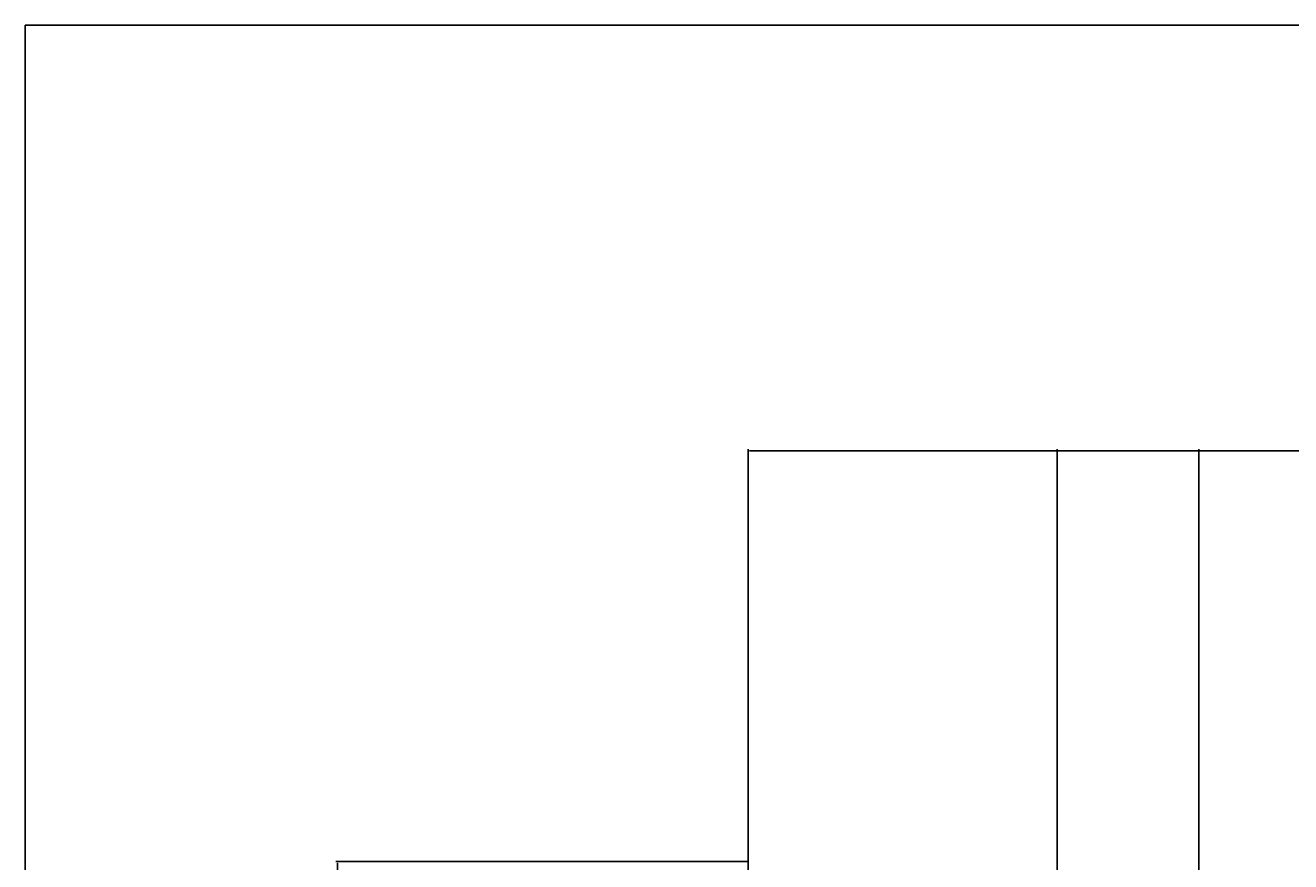
# Model space of a CAD drawing. Units: inches. Extents: x 1601 to 2297, y 1496 to 2631.
# Tile 41 of 57: x 1601 to 1750, y 2532 to 2631. Entities that reach past the tile are written whole.
import ezdxf

# ---------------------------------------------------------------- set-up
doc = ezdxf.new("R2010")
doc.units = ezdxf.units.IN
doc.layers.add('A-ANNO-DIMS', color=2, linetype='Continuous', lineweight=18)
doc.layers.add('A-ANNO-TTLB', color=7, linetype='Continuous', lineweight=25)
doc.styles.get("Standard").update_dxf_attribs({"font": 'arial.ttf'})
doc.dimstyles.get("Standard").update_dxf_attribs({"dimtxt": 0.18, "dimasz": 0.18, "dimexe": 0.18, "dimexo": 0.0625, "dimgap": 0.09, "dimtad": 0, "dimtih": 1, "dimtoh": 1, "dimdec": 4, "dimzin": 0, "dimdsep": 46, "dimtxsty": 'Standard', "dimcen": 0.09, "dimadec": 0, "dimazin": 0, "dimtfac": 1, "dimtdec": 4, "dimtofl": 0, "dimtmove": 0, "dimatfit": 3, "dimfxl": 1, "dimtolj": 1, "dimtzin": 0, "dimarcsym": 0})

# ---------------------------------------------------------------- blocks, each defined once
blk = doc.blocks.new('*D28')
at = {"layer": 'A-ANNO-DIMS', "color": 0, "lineweight": -2, "transparency": 16777216}
for p, q in [((1686.04, 2532.39), (1686.04, 2581.06)), ((1686.22, 2580.88), (1957.89, 2580.88)), ((2230.36, 2580.88), (1958.68, 2580.88)), ((2230.54, 2532.39), (2230.54, 2581.06))]:
    blk.add_line(p, q, dxfattribs=at)
at = {"layer": 'A-ANNO-DIMS', "color": 0, "transparency": 16777216}
for points in [[(1686.22, 2580.91), (1686.22, 2580.85), (1686.04, 2580.88)], [(2230.36, 2580.91), (2230.36, 2580.85), (2230.54, 2580.88)]]:
    blk.add_solid(points, dxfattribs=at)
at = {"layer": 'Defpoints', "color": 0, "transparency": 16777216}
for p in [(2230.54, 2580.88), (1686.04, 2532.33), (2230.54, 2532.33)]:
    blk.add_point(p, dxfattribs=at)
at = {"layer": 'A-ANNO-DIMS', "color": 0, "transparency": 16777216, "insert": (1958.29, 2580.88), "char_height": 0.18, "attachment_point": 5}
blk.add_mtext('\\A1;544.5', dxfattribs=at)
blk = doc.blocks.new('*D32')
at = {"layer": 'A-ANNO-DIMS', "color": 0, "lineweight": -2, "transparency": 16777216}
for p, q in [((1686.04, 2031.39), (1686.04, 2581.06)), ((1686.22, 2580.88), (1703.91, 2580.88)), ((1722.39, 2580.88), (1704.7, 2580.88)), ((1722.57, 2031.39), (1722.57, 2581.06))]:
    blk.add_line(p, q, dxfattribs=at)
at = {"layer": 'A-ANNO-DIMS', "color": 0, "transparency": 16777216}
for points in [[(1686.22, 2580.91), (1686.22, 2580.85), (1686.04, 2580.88)], [(1722.39, 2580.91), (1722.39, 2580.85), (1722.57, 2580.88)]]:
    blk.add_solid(points, dxfattribs=at)
at = {"layer": 'Defpoints', "color": 0, "transparency": 16777216}
for p in [(1722.57, 2580.88), (1686.04, 2031.33), (1722.57, 2031.33)]:
    blk.add_point(p, dxfattribs=at)
at = {"layer": 'A-ANNO-DIMS', "color": 0, "transparency": 16777216, "insert": (1704.3, 2580.88), "char_height": 0.18, "attachment_point": 5}
blk.add_mtext('\\A1;36.53', dxfattribs=at)
blk = doc.blocks.new('*D35')
at = {"layer": 'A-ANNO-DIMS', "color": 0, "lineweight": -2, "transparency": 16777216}
for p, q in [((1685.97, 2532.33), (1637.31, 2532.33)), ((1637.49, 2532.15), (1637.49, 2512.82)), ((1637.49, 2493.13), (1637.49, 2512.46)), ((1685.97, 2492.95), (1637.31, 2492.95))]:
    blk.add_line(p, q, dxfattribs=at)
at = {"layer": 'A-ANNO-DIMS', "color": 0, "transparency": 16777216}
for points in [[(1637.46, 2532.15), (1637.52, 2532.15), (1637.49, 2532.33)], [(1637.46, 2493.13), (1637.52, 2493.13), (1637.49, 2492.95)]]:
    blk.add_solid(points, dxfattribs=at)
at = {"layer": 'Defpoints', "color": 0, "transparency": 16777216}
for p in [(1637.49, 2532.33), (1686.04, 2532.33), (1686.04, 2492.95)]:
    blk.add_point(p, dxfattribs=at)
at = {"layer": 'A-ANNO-DIMS', "color": 0, "transparency": 16777216, "insert": (1637.49, 2512.64), "char_height": 0.18, "attachment_point": 5}
blk.add_mtext('\\A1;39.376', dxfattribs=at)
blk = doc.blocks.new('*D36')
at = {"layer": 'A-ANNO-DIMS', "color": 0, "lineweight": -2, "transparency": 16777216}
for p, q in [((1686.04, 1635.39), (1686.04, 2581.06)), ((1686.22, 2580.88), (1712.36, 2580.88)), ((1739.15, 2580.88), (1713.01, 2580.88)), ((1739.33, 1635.39), (1739.33, 2581.06))]:
    blk.add_line(p, q, dxfattribs=at)
at = {"layer": 'A-ANNO-DIMS', "color": 0, "transparency": 16777216}
for points in [[(1686.22, 2580.91), (1686.22, 2580.85), (1686.04, 2580.88)], [(1739.15, 2580.91), (1739.15, 2580.85), (1739.33, 2580.88)]]:
    blk.add_solid(points, dxfattribs=at)
at = {"layer": 'Defpoints', "color": 0, "transparency": 16777216}
for p in [(1739.33, 2580.88), (1686.04, 1635.33), (1739.33, 1635.33)]:
    blk.add_point(p, dxfattribs=at)
at = {"layer": 'A-ANNO-DIMS', "color": 0, "transparency": 16777216, "insert": (1712.69, 2580.88), "char_height": 0.18, "attachment_point": 5}
blk.add_mtext('\\A1;53.3', dxfattribs=at)

msp = doc.modelspace()

# ---------------------------------------------------------------- linework, layer by layer
at = {"layer": 'A-ANNO-TTLB'}
msp.add_lwpolyline([(1600.5933, 2631.1477), (2297.129, 2631.1477), (2297.129, 1496.1026), (1600.5933, 1496.1026)], close=True, dxfattribs=at)

# ---------------------------------------------------------------- dimensions: what is measured, and where the dimension line sits
at = {"layer": 'A-ANNO-DIMS'}
for base, p1, p2, override, picture, middle in [((2230.5373, 2580.8754), (1686.0373, 2532.3254), (2230.5373, 2532.3254), {"dimdec": 1, "dimlfac": 1, "dimrnd": 0, "dimzin": 0, "dimdsep": 46, "dimlunit": 2}, '*D28', (1958.2873, 2580.8754)), ((1722.5687, 2580.8754), (1686.0373, 2031.3254), (1722.5687, 2031.3254), {"dimdec": 2, "dimlfac": 1, "dimrnd": 0, "dimzin": 0, "dimdsep": 46, "dimlunit": 2}, '*D32', (1704.303, 2580.8754)), ((1739.3335, 2580.8754), (1686.0373, 1635.3254), (1739.3335, 1635.3254), {"dimdec": 1, "dimlfac": 1, "dimrnd": 0, "dimzin": 0, "dimdsep": 46, "dimlunit": 2}, '*D36', (1712.6854, 2580.8754))]:
    dim = msp.add_linear_dim(base=base, p1=p1, p2=p2, dimstyle='Standard', override=override, dxfattribs=at)
    dim.commit()
    dim.dimension.update_dxf_attribs({"geometry": picture, "text_midpoint": middle})
dim = msp.add_linear_dim(base=(1637.4873, 2532.3254), p1=(1686.0373, 2492.9493), p2=(1686.0373, 2532.3254), angle=90, dimstyle='Standard', override={"dimdec": 3, "dimlfac": 1, "dimrnd": 0, "dimzin": 0, "dimdsep": 46, "dimlunit": 2}, dxfattribs=at)
dim.commit()
dim.dimension.update_dxf_attribs({"geometry": '*D35', "text_midpoint": (1637.4873, 2512.6374)})

doc.saveas('drawing.dxf')
